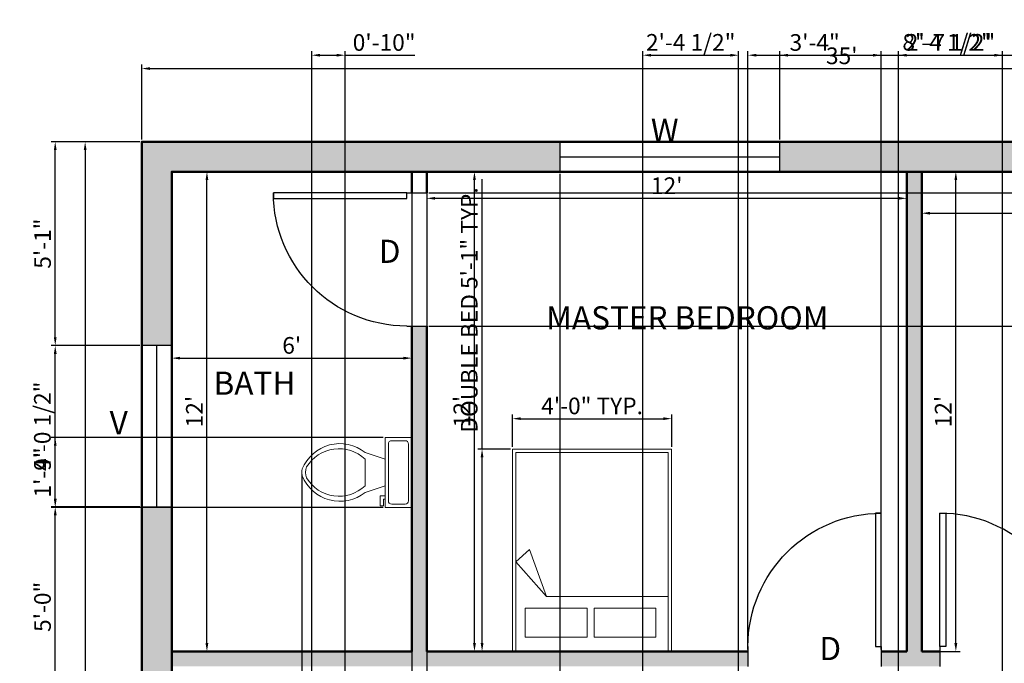
# Model space of a CAD drawing. Units: inches. Extents: x 2168 to 2706, y 2255 to 2760.
# Tile 3 of 4: x 2168 to 2463, y 2567 to 2760. Entities that reach past the tile are written whole.
import ezdxf

# ---------------------------------------------------------------- set-up
doc = ezdxf.new("R2010")
doc.units = ezdxf.units.IN
for name, color, linetype, lineweight in [('A-ANNO-DIMS', 220, 'Continuous', 18), ('A-ANNO-TEXT', 220, 'Continuous', 25), ('A-AREA-IDEN', 220, 'Continuous', 25), ('A-FLOR-FIXT', 9, 'Continuous', 18), ('A-WALL-PATT', 140, 'Continuous', 13), ('DOOR', 30, 'Continuous', 25), ('FUR', 112, 'Continuous', 18), ('WALL', 140, 'Continuous', 50), ('WINDOW', 200, 'Continuous', 25)]:
    doc.layers.add(name, color=color, linetype=linetype, lineweight=lineweight)
doc.styles.get("Standard").update_dxf_attribs({"font": 'arial.ttf'})
doc.dimstyles.new('ISO-25', dxfattribs={"dimtxt": 5, "dimasz": 2.5, "dimexe": 1.25, "dimexo": 0.625, "dimtad": 1, "dimlunit": 4, "dimtxsty": 'Standard', "dimcen": 2.5, "dimadec": 0, "dimazin": 0, "dimtfac": 1, "dimtmove": 0, "dimatfit": 3, "dimfxl": 1, "dimarcsym": 0})

# ---------------------------------------------------------------- blocks, each defined once
blk = doc.blocks.new('*U2')
for p, q in [((0, 0), (0, -6)), ((40, 0), (40, -6))]:
    blk.add_line(p, q)
blk.add_lwpolyline([(0, 0), (0, 40), (1.75, 40), (1.75, 0)], close=True)
blk.add_arc((0, 0), 40, 0, 90)
blk = doc.blocks.new('*U4')
for p, q in [((9.5, -6), (9.5, -2)), ((-10, -8.5), (-8, -8.5)), ((-10, -9.5), (-10, -8.5)), ((-8, -8.5), (-8, -8)), ((-7, -8), (-7, -9.5)), ((-4, -8), (-6, -14)), ((4, -8), (6, -14)), ((-7, -9.5), (-10, -9.5)), ((4, -14), (-4, -14))]:
    blk.add_line(p, q)
blk.add_lwpolyline([(10.5, -8), (10.5, 0), (-10.5, 0), (-10.5, -8)], close=True)
for points in [[(-9.5, -2), (-9.5, -6)], [(8.5, -1), (-8.5, -1)], [(-8.5, -7), (8.5, -7)]]:
    blk.add_lwpolyline(points)
for centre, radius, start, end in [((-8.62, -1.88), 0.884, 81.8699, 188.1301), ((8.62, -1.88), 0.884, 351.8699, 98.1301), ((-8.62, -6.12), 0.884, 171.8699, 278.1301), ((8.62, -6.12), 0.884, 261.8699, 8.1301), ((3.52, -21.58), 12.17, 141.4691, 247.9714), ((4.2, -21.82), 11.33, 136.3677, 238.9468), ((-3.52, -21.58), 12.17, 292.0284, 38.5307), ((-4.2, -21.82), 11.33, 301.053, 43.6321), ((0, -27.88), 4, 245.7318, 294.2682), ((0, -29), 4, 254.8605, 285.1395)]:
    blk.add_arc(centre, radius, start, end)
blk = doc.blocks.new('*D5')
at = {"layer": 'A-ANNO-DIMS', "color": 0, "lineweight": -2, "transparency": 16777216}
for p, q in [((2213.72, 2713.72), (2213.72, 2657.14)), ((2285.72, 2713.72), (2285.72, 2657.14)), ((2216.22, 2658.39), (2283.22, 2658.39))]:
    blk.add_line(p, q, dxfattribs=at)
at = {"layer": 'A-ANNO-DIMS', "color": 0, "transparency": 16777216}
for points in [[(2216.22, 2658.8), (2216.22, 2657.97), (2213.72, 2658.39)], [(2283.22, 2658.8), (2283.22, 2657.97), (2285.72, 2658.39)]]:
    blk.add_solid(points, dxfattribs=at)
at = {"layer": 'Defpoints', "color": 0, "transparency": 16777216}
for p in [(2213.72, 2714.35), (2285.72, 2714.35), (2285.72, 2658.39)]:
    blk.add_point(p, dxfattribs=at)
at = {"layer": 'A-ANNO-DIMS', "color": 0, "transparency": 16777216, "insert": (2249.72, 2661.56), "char_height": 5, "attachment_point": 5}
blk.add_mtext("6'", dxfattribs=at)
blk = doc.blocks.new('*D6')
at = {"layer": 'A-ANNO-DIMS', "color": 0, "lineweight": -2, "transparency": 16777216}
for p, q in [((2214.35, 2714.35), (2225.53, 2714.35)), ((2224.28, 2572.85), (2224.28, 2711.85)), ((2214.35, 2570.35), (2225.53, 2570.35))]:
    blk.add_line(p, q, dxfattribs=at)
at = {"layer": 'A-ANNO-DIMS', "color": 0, "transparency": 16777216}
for points in [[(2223.86, 2711.85), (2224.7, 2711.85), (2224.28, 2714.35)], [(2223.86, 2572.85), (2224.7, 2572.85), (2224.28, 2570.35)]]:
    blk.add_solid(points, dxfattribs=at)
at = {"layer": 'Defpoints', "color": 0, "transparency": 16777216}
for p in [(2213.72, 2714.35), (2224.28, 2714.35), (2213.72, 2570.35)]:
    blk.add_point(p, dxfattribs=at)
at = {"layer": 'A-ANNO-DIMS', "color": 0, "transparency": 16777216, "insert": (2221.15, 2642.35), "char_height": 5, "attachment_point": 5, "rotation": 90}
blk.add_mtext("12'", dxfattribs=at)
blk = doc.blocks.new('*D7')
at = {"layer": 'A-ANNO-DIMS', "color": 0, "lineweight": -2, "transparency": 16777216}
for p, q in [((2290.22, 2713.72), (2290.22, 2705.1)), ((2434.22, 2713.72), (2434.22, 2705.1)), ((2292.72, 2706.35), (2431.72, 2706.35))]:
    blk.add_line(p, q, dxfattribs=at)
at = {"layer": 'A-ANNO-DIMS', "color": 0, "transparency": 16777216}
for points in [[(2292.72, 2706.77), (2292.72, 2705.93), (2290.22, 2706.35)], [(2431.72, 2706.77), (2431.72, 2705.93), (2434.22, 2706.35)]]:
    blk.add_solid(points, dxfattribs=at)
at = {"layer": 'Defpoints', "color": 0, "transparency": 16777216}
for p in [(2290.22, 2714.35), (2434.22, 2714.35), (2434.22, 2706.35)]:
    blk.add_point(p, dxfattribs=at)
at = {"layer": 'A-ANNO-DIMS', "color": 0, "transparency": 16777216, "insert": (2362.22, 2709.49), "char_height": 5, "attachment_point": 5}
blk.add_mtext("12'", dxfattribs=at)
blk = doc.blocks.new('*D8')
at = {"layer": 'A-ANNO-DIMS', "color": 0, "lineweight": -2, "transparency": 16777216}
for p, q in [((2290.85, 2714.35), (2305.79, 2714.35)), ((2304.54, 2572.85), (2304.54, 2711.85)), ((2290.85, 2570.35), (2305.79, 2570.35))]:
    blk.add_line(p, q, dxfattribs=at)
at = {"layer": 'A-ANNO-DIMS', "color": 0, "transparency": 16777216}
for points in [[(2304.12, 2711.85), (2304.95, 2711.85), (2304.54, 2714.35)], [(2304.12, 2572.85), (2304.95, 2572.85), (2304.54, 2570.35)]]:
    blk.add_solid(points, dxfattribs=at)
at = {"layer": 'Defpoints', "color": 0, "transparency": 16777216}
for p in [(2290.22, 2714.35), (2304.54, 2714.35), (2290.22, 2570.35)]:
    blk.add_point(p, dxfattribs=at)
at = {"layer": 'A-ANNO-DIMS', "color": 0, "transparency": 16777216, "insert": (2301.4, 2642.35), "char_height": 5, "attachment_point": 5, "rotation": 90}
blk.add_mtext("12'", dxfattribs=at)
blk = doc.blocks.new('*D9')
at = {"layer": 'A-ANNO-DIMS', "color": 0, "lineweight": -2, "transparency": 16777216}
for p, q in [((2438.72, 2713.72), (2438.72, 2700.63)), ((2615.72, 2713.72), (2615.72, 2700.63)), ((2441.22, 2701.88), (2613.22, 2701.88))]:
    blk.add_line(p, q, dxfattribs=at)
at = {"layer": 'A-ANNO-DIMS', "color": 0, "transparency": 16777216}
for points in [[(2441.22, 2702.3), (2441.22, 2701.46), (2438.72, 2701.88)], [(2613.22, 2702.3), (2613.22, 2701.46), (2615.72, 2701.88)]]:
    blk.add_solid(points, dxfattribs=at)
at = {"layer": 'Defpoints', "color": 0, "transparency": 16777216}
for p in [(2438.72, 2714.35), (2615.72, 2714.35), (2615.72, 2701.88)]:
    blk.add_point(p, dxfattribs=at)
at = {"layer": 'A-ANNO-DIMS', "color": 0, "transparency": 16777216, "insert": (2527.22, 2705.06), "char_height": 5, "attachment_point": 5}
blk.add_mtext('14\'-9"', dxfattribs=at)
blk = doc.blocks.new('*D10')
at = {"layer": 'A-ANNO-DIMS', "color": 0, "lineweight": -2, "transparency": 16777216}
for p, q in [((2439.35, 2714.35), (2450.2, 2714.35)), ((2448.95, 2572.85), (2448.95, 2711.85)), ((2439.35, 2570.35), (2450.2, 2570.35))]:
    blk.add_line(p, q, dxfattribs=at)
at = {"layer": 'A-ANNO-DIMS', "color": 0, "transparency": 16777216}
for points in [[(2448.53, 2711.85), (2449.37, 2711.85), (2448.95, 2714.35)], [(2448.53, 2572.85), (2449.37, 2572.85), (2448.95, 2570.35)]]:
    blk.add_solid(points, dxfattribs=at)
at = {"layer": 'Defpoints', "color": 0, "transparency": 16777216}
for p in [(2438.72, 2714.35), (2448.95, 2714.35), (2438.72, 2570.35)]:
    blk.add_point(p, dxfattribs=at)
at = {"layer": 'A-ANNO-DIMS', "color": 0, "transparency": 16777216, "insert": (2445.81, 2642.35), "char_height": 5, "attachment_point": 5, "rotation": 90}
blk.add_mtext("12'", dxfattribs=at)
blk = doc.blocks.new('*D29')
at = {"layer": 'A-ANNO-DIMS', "color": 0, "lineweight": -2, "transparency": 16777216}
for p, q in [((2204.72, 2723.97), (2204.72, 2746.55)), ((2207.22, 2745.3), (2622.22, 2745.3)), ((2624.72, 2723.97), (2624.72, 2746.55))]:
    blk.add_line(p, q, dxfattribs=at)
at = {"layer": 'A-ANNO-DIMS', "color": 0, "transparency": 16777216}
for points in [[(2207.22, 2745.71), (2207.22, 2744.88), (2204.72, 2745.3)], [(2622.22, 2745.71), (2622.22, 2744.88), (2624.72, 2745.3)]]:
    blk.add_solid(points, dxfattribs=at)
at = {"layer": 'Defpoints', "color": 0, "transparency": 16777216}
for p in [(2624.72, 2745.3), (2204.72, 2723.35), (2624.72, 2723.35)]:
    blk.add_point(p, dxfattribs=at)
at = {"layer": 'A-ANNO-DIMS', "color": 0, "transparency": 16777216, "insert": (2414.72, 2748.48), "char_height": 5, "attachment_point": 5}
blk.add_mtext("35'", dxfattribs=at)
blk = doc.blocks.new('*D30')
at = {"layer": 'A-ANNO-DIMS', "color": 0, "lineweight": -2, "transparency": 16777216}
for p, q in [((2204.1, 2723.35), (2186.49, 2723.35)), ((2187.74, 2720.85), (2187.74, 2305.85)), ((2204.1, 2303.35), (2186.49, 2303.35))]:
    blk.add_line(p, q, dxfattribs=at)
at = {"layer": 'A-ANNO-DIMS', "color": 0, "transparency": 16777216}
for points in [[(2187.33, 2720.85), (2188.16, 2720.85), (2187.74, 2723.35)], [(2187.33, 2305.85), (2188.16, 2305.85), (2187.74, 2303.35)]]:
    blk.add_solid(points, dxfattribs=at)
at = {"layer": 'Defpoints', "color": 0, "transparency": 16777216}
for p in [(2204.72, 2723.35), (2187.74, 2303.35), (2204.72, 2303.35)]:
    blk.add_point(p, dxfattribs=at)
at = {"layer": 'A-ANNO-DIMS', "color": 0, "transparency": 16777216, "insert": (2184.56, 2513.35), "char_height": 5, "attachment_point": 5, "rotation": 90}
blk.add_mtext("35'", dxfattribs=at)
blk = doc.blocks.new('BED-DOUBLE')
for p, q in [((0, 26.86), (4.14, 30.57)), ((4.14, 30.57), (9.23, 16.54)), ((9.23, 16.54), (0, 26.86)), ((45.76, 16.54), (9.23, 16.54))]:
    blk.add_line(p, q)
blk.add_lwpolyline([(46.76, 0), (46.76, 60.76), (-1, 60.76), (-1, 0)])
for points in [[(0, 0), (45.76, 0), (45.76, 59.76), (0, 59.76)], [(2.85, 4.25), (21.39, 4.25), (21.39, 13.05), (2.85, 13.05)], [(23.51, 4.25), (42.05, 4.25), (42.05, 13.05), (23.51, 13.05)]]:
    blk.add_lwpolyline(points, close=True)
blk = doc.blocks.new('WIN-66IN')
blk.add_line((0, 0), (66.01, 0))
blk.add_lwpolyline([(0, -4.5), (66.01, -4.5), (66.01, 4.5), (0, 4.5)], close=True)
blk = doc.blocks.new('*D36')
at = {"layer": 'A-ANNO-DIMS', "color": 0, "lineweight": -2, "transparency": 16777216}
for p, q in [((2306.82, 2631.11), (2306.82, 2712.06)), ((2315.31, 2631.11), (2305.57, 2631.11)), ((2306.82, 2572.85), (2306.82, 2628.61)), ((2315.31, 2570.35), (2305.57, 2570.35))]:
    blk.add_line(p, q, dxfattribs=at)
at = {"layer": 'A-ANNO-DIMS', "color": 0, "transparency": 16777216}
for points in [[(2306.4, 2628.61), (2307.24, 2628.61), (2306.82, 2631.11)], [(2306.4, 2572.85), (2307.24, 2572.85), (2306.82, 2570.35)]]:
    blk.add_solid(points, dxfattribs=at)
at = {"layer": 'Defpoints', "color": 0, "transparency": 16777216}
for p in [(2306.82, 2631.11), (2315.94, 2631.11), (2315.94, 2570.35)]:
    blk.add_point(p, dxfattribs=at)
at = {"layer": 'A-ANNO-DIMS', "color": 0, "transparency": 16777216, "insert": (2303.61, 2672.83), "char_height": 5, "attachment_point": 5, "rotation": 90}
blk.add_mtext('DOUBLE BED 5\'-1" TYP.', dxfattribs=at)
blk = doc.blocks.new('*D37')
at = {"layer": 'A-ANNO-DIMS', "color": 0, "lineweight": -2, "transparency": 16777216}
for p, q in [((2315.94, 2631.74), (2315.94, 2641.47)), ((2363.7, 2631.74), (2363.7, 2641.47)), ((2318.44, 2640.22), (2361.2, 2640.22))]:
    blk.add_line(p, q, dxfattribs=at)
at = {"layer": 'A-ANNO-DIMS', "color": 0, "transparency": 16777216}
for points in [[(2318.44, 2640.64), (2318.44, 2639.81), (2315.94, 2640.22)], [(2361.2, 2640.64), (2361.2, 2639.81), (2363.7, 2640.22)]]:
    blk.add_solid(points, dxfattribs=at)
at = {"layer": 'Defpoints', "color": 0, "transparency": 16777216}
for p in [(2363.7, 2640.22), (2315.94, 2631.11), (2363.7, 2631.11)]:
    blk.add_point(p, dxfattribs=at)
at = {"layer": 'A-ANNO-DIMS', "color": 0, "transparency": 16777216, "insert": (2339.82, 2643.4), "char_height": 5, "attachment_point": 5}
blk.add_mtext('4\'-0" TYP.', dxfattribs=at)
blk = doc.blocks.new('*D47')
at = {"layer": 'A-ANNO-DIMS', "color": 0, "lineweight": -2, "transparency": 16777216}
for p, q in [((2386.59, 2570.97), (2386.59, 2750.55)), ((2426.59, 2570.97), (2426.59, 2750.55)), ((2389.09, 2749.3), (2424.09, 2749.3))]:
    blk.add_line(p, q, dxfattribs=at)
at = {"layer": 'A-ANNO-DIMS', "color": 0, "transparency": 16777216}
for points in [[(2389.09, 2749.71), (2389.09, 2748.88), (2386.59, 2749.3)], [(2424.09, 2749.71), (2424.09, 2748.88), (2426.59, 2749.3)]]:
    blk.add_solid(points, dxfattribs=at)
at = {"layer": 'Defpoints', "color": 0, "transparency": 16777216}
for p in [(2426.59, 2749.3), (2386.59, 2570.35), (2426.59, 2570.35)]:
    blk.add_point(p, dxfattribs=at)
at = {"layer": 'A-ANNO-DIMS', "color": 0, "transparency": 16777216, "insert": (2406.59, 2752.48), "char_height": 5, "attachment_point": 5}
blk.add_mtext('3\'-4"', dxfattribs=at)
blk = doc.blocks.new('*D49')
at = {"layer": 'A-ANNO-DIMS', "color": 0, "lineweight": -2, "transparency": 16777216}
for p, q in [((2355.04, 2389.47), (2355.04, 2750.55)), ((2383.78, 2389.47), (2383.78, 2750.55)), ((2357.54, 2749.3), (2381.28, 2749.3))]:
    blk.add_line(p, q, dxfattribs=at)
at = {"layer": 'A-ANNO-DIMS', "color": 0, "transparency": 16777216}
for points in [[(2357.54, 2749.71), (2357.54, 2748.88), (2355.04, 2749.3)], [(2381.28, 2749.71), (2381.28, 2748.88), (2383.78, 2749.3)]]:
    blk.add_solid(points, dxfattribs=at)
at = {"layer": 'Defpoints', "color": 0, "transparency": 16777216}
for p in [(2383.78, 2749.3), (2355.04, 2388.85), (2383.78, 2388.85)]:
    blk.add_point(p, dxfattribs=at)
at = {"layer": 'A-ANNO-DIMS', "color": 0, "transparency": 16777216, "insert": (2369.41, 2752.51), "char_height": 5, "attachment_point": 5}
blk.add_mtext('2\'-4 1/2"', dxfattribs=at)
blk = doc.blocks.new('*D53')
at = {"layer": 'A-ANNO-DIMS', "color": 0, "lineweight": -2, "transparency": 16777216}
for p, q in [((2431.71, 2524.6), (2431.71, 2750.55)), ((2462.98, 2524.6), (2462.98, 2750.55)), ((2434.21, 2749.3), (2460.48, 2749.3))]:
    blk.add_line(p, q, dxfattribs=at)
at = {"layer": 'A-ANNO-DIMS', "color": 0, "transparency": 16777216}
for points in [[(2434.21, 2749.71), (2434.21, 2748.88), (2431.71, 2749.3)], [(2460.48, 2749.71), (2460.48, 2748.88), (2462.98, 2749.3)]]:
    blk.add_solid(points, dxfattribs=at)
at = {"layer": 'Defpoints', "color": 0, "transparency": 16777216}
for p in [(2462.98, 2749.3), (2431.71, 2523.98), (2462.98, 2523.98)]:
    blk.add_point(p, dxfattribs=at)
at = {"layer": 'A-ANNO-DIMS', "color": 0, "transparency": 16777216, "insert": (2447.34, 2752.51), "char_height": 5, "attachment_point": 5}
blk.add_mtext('2\'-7 1/2"', dxfattribs=at)
blk = doc.blocks.new('*D64')
at = {"layer": 'A-ANNO-DIMS', "color": 0, "lineweight": -2, "transparency": 16777216}
for p, q in [((2290.22, 2713.72), (2290.22, 2276.15)), ((2330.12, 2713.72), (2330.12, 2276.15)), ((2292.72, 2277.4), (2327.62, 2277.4))]:
    blk.add_line(p, q, dxfattribs=at)
at = {"layer": 'A-ANNO-DIMS', "color": 0, "transparency": 16777216}
for points in [[(2292.72, 2277.81), (2292.72, 2276.98), (2290.22, 2277.4)], [(2327.62, 2277.81), (2327.62, 2276.98), (2330.12, 2277.4)]]:
    blk.add_solid(points, dxfattribs=at)
at = {"layer": 'Defpoints', "color": 0, "transparency": 16777216}
for p in [(2290.22, 2714.35), (2330.12, 2714.35), (2330.12, 2277.4)]:
    blk.add_point(p, dxfattribs=at)
at = {"layer": 'A-ANNO-DIMS', "color": 0, "transparency": 16777216, "insert": (2310.17, 2280.58), "char_height": 5, "attachment_point": 5}
blk.add_mtext('3\'-4"', dxfattribs=at)
blk = doc.blocks.new('*D65')
at = {"layer": 'A-ANNO-DIMS', "color": 0, "lineweight": -2, "transparency": 16777216}
for p, q in [((2396.13, 2723.97), (2396.13, 2750.55)), ((2496.54, 2723.97), (2496.54, 2750.55)), ((2398.63, 2749.3), (2494.04, 2749.3))]:
    blk.add_line(p, q, dxfattribs=at)
at = {"layer": 'A-ANNO-DIMS', "color": 0, "transparency": 16777216}
for points in [[(2398.63, 2749.71), (2398.63, 2748.88), (2396.13, 2749.3)], [(2494.04, 2749.71), (2494.04, 2748.88), (2496.54, 2749.3)]]:
    blk.add_solid(points, dxfattribs=at)
at = {"layer": 'Defpoints', "color": 0, "transparency": 16777216}
for p in [(2496.54, 2749.3), (2396.13, 2723.35), (2496.54, 2723.35)]:
    blk.add_point(p, dxfattribs=at)
at = {"layer": 'A-ANNO-DIMS', "color": 0, "transparency": 16777216, "insert": (2446.33, 2752.51), "char_height": 5, "attachment_point": 5}
blk.add_mtext('8\'-4 1/2"', dxfattribs=at)
blk = doc.blocks.new('*D68')
at = {"layer": 'A-ANNO-DIMS', "color": 0, "lineweight": -2, "transparency": 16777216}
for p, q in [((2204.1, 2662.15), (2177.52, 2662.15)), ((2178.77, 2616.23), (2178.77, 2659.65)), ((2204.1, 2613.73), (2177.52, 2613.73))]:
    blk.add_line(p, q, dxfattribs=at)
at = {"layer": 'A-ANNO-DIMS', "color": 0, "transparency": 16777216}
for points in [[(2178.36, 2659.65), (2179.19, 2659.65), (2178.77, 2662.15)], [(2178.36, 2616.23), (2179.19, 2616.23), (2178.77, 2613.73)]]:
    blk.add_solid(points, dxfattribs=at)
at = {"layer": 'Defpoints', "color": 0, "transparency": 16777216}
for p in [(2178.77, 2662.15), (2204.72, 2662.15), (2204.72, 2613.73)]:
    blk.add_point(p, dxfattribs=at)
at = {"layer": 'A-ANNO-DIMS', "color": 0, "transparency": 16777216, "insert": (2175.56, 2637.94), "char_height": 5, "attachment_point": 5, "rotation": 90}
blk.add_mtext('4\'-0 1/2"', dxfattribs=at)
blk = doc.blocks.new('*D69')
at = {"layer": 'A-ANNO-DIMS', "color": 0, "lineweight": -2, "transparency": 16777216}
for p, q in [((2204.1, 2723.35), (2177.52, 2723.35)), ((2178.77, 2664.65), (2178.77, 2720.85)), ((2204.1, 2662.15), (2177.52, 2662.15))]:
    blk.add_line(p, q, dxfattribs=at)
at = {"layer": 'A-ANNO-DIMS', "color": 0, "transparency": 16777216}
for points in [[(2178.36, 2720.85), (2179.19, 2720.85), (2178.77, 2723.35)], [(2178.36, 2664.65), (2179.19, 2664.65), (2178.77, 2662.15)]]:
    blk.add_solid(points, dxfattribs=at)
at = {"layer": 'Defpoints', "color": 0, "transparency": 16777216}
for p in [(2178.77, 2723.35), (2204.72, 2723.35), (2204.72, 2662.15)]:
    blk.add_point(p, dxfattribs=at)
at = {"layer": 'A-ANNO-DIMS', "color": 0, "transparency": 16777216, "insert": (2175.6, 2692.75), "char_height": 5, "attachment_point": 5, "rotation": 90}
blk.add_mtext('5\'-1"', dxfattribs=at)
blk = doc.blocks.new('*D71')
at = {"layer": 'A-ANNO-DIMS', "color": 0, "lineweight": -2, "transparency": 16777216}
for p, q in [((2204.1, 2613.73), (2177.52, 2613.73)), ((2178.77, 2556.26), (2178.77, 2611.23)), ((2204.1, 2553.76), (2177.52, 2553.76))]:
    blk.add_line(p, q, dxfattribs=at)
at = {"layer": 'A-ANNO-DIMS', "color": 0, "transparency": 16777216}
for points in [[(2178.36, 2611.23), (2179.19, 2611.23), (2178.77, 2613.73)], [(2178.36, 2556.26), (2179.19, 2556.26), (2178.77, 2553.76)]]:
    blk.add_solid(points, dxfattribs=at)
at = {"layer": 'Defpoints', "color": 0, "transparency": 16777216}
for p in [(2178.77, 2613.73), (2204.72, 2613.73), (2204.72, 2553.76)]:
    blk.add_point(p, dxfattribs=at)
at = {"layer": 'A-ANNO-DIMS', "color": 0, "transparency": 16777216, "insert": (2175.6, 2583.75), "char_height": 5, "attachment_point": 5, "rotation": 90}
blk.add_mtext('5\'-0"', dxfattribs=at)
blk = doc.blocks.new('*D74')
at = {"layer": 'A-ANNO-DIMS', "color": 0, "lineweight": -2, "transparency": 16777216}
for p, q in [((2255.72, 2525.22), (2255.72, 2750.55)), ((2265.72, 2525.22), (2265.72, 2750.55)), ((2258.22, 2749.3), (2263.22, 2749.3)), ((2265.72, 2749.3), (2286.65, 2749.3))]:
    blk.add_line(p, q, dxfattribs=at)
at = {"layer": 'A-ANNO-DIMS', "color": 0, "transparency": 16777216}
for points in [[(2258.22, 2749.71), (2258.22, 2748.88), (2255.72, 2749.3)], [(2263.22, 2749.71), (2263.22, 2748.88), (2265.72, 2749.3)]]:
    blk.add_solid(points, dxfattribs=at)
at = {"layer": 'Defpoints', "color": 0, "transparency": 16777216}
for p in [(2265.72, 2749.3), (2255.72, 2524.6), (2265.72, 2524.6)]:
    blk.add_point(p, dxfattribs=at)
at = {"layer": 'A-ANNO-DIMS', "color": 0, "transparency": 16777216, "insert": (2277.44, 2752.47), "char_height": 5, "attachment_point": 5}
blk.add_mtext('0\'-10"', dxfattribs=at)
blk = doc.blocks.new('*D75')
at = {"layer": 'A-ANNO-DIMS', "color": 0, "lineweight": -2, "transparency": 16777216}
for p, q in [((2277.1, 2634.58), (2177.52, 2634.58)), ((2178.77, 2616.08), (2178.77, 2632.08)), ((2277.1, 2613.58), (2177.52, 2613.58))]:
    blk.add_line(p, q, dxfattribs=at)
at = {"layer": 'A-ANNO-DIMS', "color": 0, "transparency": 16777216}
for points in [[(2178.36, 2632.08), (2179.19, 2632.08), (2178.77, 2634.58)], [(2178.36, 2616.08), (2179.19, 2616.08), (2178.77, 2613.58)]]:
    blk.add_solid(points, dxfattribs=at)
at = {"layer": 'Defpoints', "color": 0, "transparency": 16777216}
for p in [(2178.77, 2634.58), (2277.72, 2634.58), (2277.72, 2613.58)]:
    blk.add_point(p, dxfattribs=at)
at = {"layer": 'A-ANNO-DIMS', "color": 0, "transparency": 16777216, "insert": (2175.6, 2624.08), "char_height": 5, "attachment_point": 5, "rotation": 90}
blk.add_mtext('1\'-9"', dxfattribs=at)
blk = doc.blocks.new('*D76')
at = {"layer": 'A-ANNO-DIMS', "color": 0, "lineweight": -2, "transparency": 16777216}
for p, q in [((2252.72, 2623.46), (2252.72, 2276.15)), ((2285.72, 2612.95), (2285.72, 2276.15)), ((2255.22, 2277.4), (2283.22, 2277.4))]:
    blk.add_line(p, q, dxfattribs=at)
at = {"layer": 'A-ANNO-DIMS', "color": 0, "transparency": 16777216}
for points in [[(2255.22, 2277.81), (2255.22, 2276.98), (2252.72, 2277.4)], [(2283.22, 2277.81), (2283.22, 2276.98), (2285.72, 2277.4)]]:
    blk.add_solid(points, dxfattribs=at)
at = {"layer": 'Defpoints', "color": 0, "transparency": 16777216}
for p in [(2252.72, 2624.08), (2285.72, 2613.58), (2285.72, 2277.4)]:
    blk.add_point(p, dxfattribs=at)
at = {"layer": 'A-ANNO-DIMS', "color": 0, "transparency": 16777216, "insert": (2269.22, 2280.57), "char_height": 5, "attachment_point": 5}
blk.add_mtext('2\'-9"', dxfattribs=at)
blk = doc.blocks.new('*D77')
at = {"layer": 'A-ANNO-DIMS', "color": 0, "lineweight": -2, "transparency": 16777216}
for p, q in [((2290.85, 2708.02), (2702.92, 2708.02)), ((2701.67, 2670.52), (2701.67, 2705.52)), ((2290.85, 2668.02), (2702.92, 2668.02))]:
    blk.add_line(p, q, dxfattribs=at)
at = {"layer": 'A-ANNO-DIMS', "color": 0, "transparency": 16777216}
for points in [[(2701.26, 2705.52), (2702.09, 2705.52), (2701.67, 2708.02)], [(2701.26, 2670.52), (2702.09, 2670.52), (2701.67, 2668.02)]]:
    blk.add_solid(points, dxfattribs=at)
at = {"layer": 'Defpoints', "color": 0, "transparency": 16777216}
for p in [(2290.22, 2708.02), (2701.67, 2708.02), (2290.22, 2668.02)]:
    blk.add_point(p, dxfattribs=at)
at = {"layer": 'A-ANNO-DIMS', "color": 0, "transparency": 16777216, "insert": (2698.49, 2688.02), "char_height": 5, "attachment_point": 5, "rotation": 90}
blk.add_mtext('3\'-4"', dxfattribs=at)

msp = doc.modelspace()

# ---------------------------------------------------------------- hatches: boundary and pattern name
at = {"layer": 'A-WALL-PATT'}
h = msp.add_hatch(color=256, dxfattribs=at)
h.dxf.hatch_style = 1
h.paths.add_polyline_path([(2330.12, 2723.347), (2204.724, 2723.347), (2204.724, 2662.147), (2213.724, 2662.147), (2213.724, 2714.347), (2285.724, 2714.347), (2330.12, 2714.347)])
h.paths.add_polyline_path([(2496.542, 2723.347), (2396.128, 2723.347), (2396.128, 2714.347), (2434.224, 2714.347), (2496.542, 2714.347)])
h.paths.add_polyline_path([(2624.724, 2723.347), (2562.55, 2723.347), (2562.55, 2714.347), (2615.724, 2714.347), (2615.724, 2545.448), (2624.724, 2545.448)])
h.paths.add_polyline_path([(2438.724, 2714.347), (2434.224, 2714.347), (2434.224, 2570.347), (2426.591, 2570.347), (2426.591, 2565.847), (2438.724, 2565.847), (2444.149, 2565.847), (2444.149, 2570.347), (2438.724, 2570.347)])
h.paths.add_polyline_path([(2290.224, 2668.023), (2285.724, 2668.023), (2285.724, 2570.347), (2213.724, 2570.347), (2213.724, 2565.847), (2290.224, 2565.847), (2386.591, 2565.847), (2386.591, 2570.347), (2290.224, 2570.347)])
h.paths.add_polyline_path([(2514.678, 2570.347), (2514.678, 2630.11), (2560.439, 2630.11), (2560.439, 2570.347)], flags=16)
h.paths.add_polyline_path([(2517.528, 2574.595), (2517.528, 2583.399), (2536.063, 2583.399), (2536.063, 2574.595)], flags=0)
h.paths.add_polyline_path([(2523.909, 2586.89), (2514.678, 2597.212), (2518.822, 2600.918)], flags=0)
h.paths.add_polyline_path([(2538.189, 2574.595), (2538.189, 2583.399), (2556.724, 2583.399), (2556.724, 2574.595)], flags=0)
h.paths.add_polyline_path([(2560.439, 2630.11), (2560.439, 2570.347), (2514.678, 2570.347), (2514.678, 2630.11)])
h.paths.add_polyline_path([(2213.724, 2389.588), (2204.724, 2389.588), (2204.724, 2303.347), (2229.06, 2303.347), (2229.06, 2312.347), (2213.724, 2312.347)])
h.paths.add_polyline_path([(2213.724, 2507.677), (2204.724, 2507.677), (2204.724, 2462.696), (2213.724, 2462.696)])
h.paths.add_polyline_path([(2204.724, 2553.759), (2213.724, 2553.759), (2213.724, 2613.731), (2204.724, 2613.731)])

# ---------------------------------------------------------------- linework, layer by layer
at = {"layer": 'WALL'}
for p, q in [((2204.724, 2723.347), (2624.724, 2723.347)), ((2204.724, 2303.347), (2204.724, 2723.347)), ((2213.724, 2714.347), (2285.724, 2714.347)), ((2285.724, 2714.347), (2285.724, 2708.023)), ((2290.224, 2714.347), (2290.224, 2708.023)), ((2290.224, 2714.347), (2434.224, 2714.347)), ((2434.224, 2714.347), (2434.224, 2570.347)), ((2438.724, 2714.347), (2438.724, 2570.347)), ((2285.724, 2668.023), (2285.724, 2570.347)), ((2290.224, 2668.023), (2290.224, 2570.347)), ((2285.724, 2570.347), (2213.724, 2570.347)), ((2386.591, 2570.347), (2290.224, 2570.347)), ((2434.224, 2570.347), (2426.591, 2570.347)), ((2438.724, 2570.347), (2444.149, 2570.347))]:
    msp.add_line(p, q, dxfattribs=at)
for points in [[(2572.054, 2303.347), (2204.724, 2303.347), (2204.724, 2723.347), (2624.724, 2723.347), (2624.724, 2303.347), (2612.054, 2303.347)], [(2572.166, 2312.347), (2213.724, 2312.347), (2213.724, 2714.347), (2615.724, 2714.347), (2615.724, 2312.347), (2610.304, 2312.347)]]:
    msp.add_lwpolyline(points, dxfattribs=at)
at = {"layer": 'WINDOW'}
msp.add_line((2209.224, 2613.731), (2209.224, 2662.147), dxfattribs=at)
msp.add_lwpolyline([(2213.724, 2662.147), (2204.724, 2662.147), (2204.724, 2613.731), (2213.724, 2613.731)], close=True, dxfattribs=at)

# ---------------------------------------------------------------- block references
at = {"layer": 'A-FLOR-FIXT', "xscale": -1, "rotation": 270}
msp.add_blockref('*U4', (2285.724, 2624.08), dxfattribs=at)
at = {"layer": 'DOOR', "xscale": -1, "rotation": 90}
msp.add_blockref('*U2', (2284.224, 2708.023), dxfattribs=at)
at = {"layer": 'DOOR', "xscale": -1}
msp.add_blockref('*U2', (2426.591, 2571.847), dxfattribs=at)
at = {"layer": 'DOOR'}
msp.add_blockref('*U2', (2444.149, 2571.847), dxfattribs=at)
at = {"layer": 'FUR'}
msp.add_blockref('BED-DOUBLE', (2316.936, 2570.347), dxfattribs=at)
at = {"layer": 'WINDOW'}
msp.add_blockref('WIN-66IN', (2330.12, 2718.847), dxfattribs=at)

# ---------------------------------------------------------------- texts
at = {"layer": 'A-ANNO-TEXT', "char_height": 6.951, "attachment_point": 1}
for s, insert in [('W', (2357.454, 2730.298)), ('D', (2275.821, 2693.919)), ('V', (2195.081, 2642.506)), ('D', (2408.003, 2574.701))]:
    msp.add_mtext_dynamic_manual_height_columns(s, width=121.01281, gutter_width=34.753, heights=[0], dxfattribs=dict(at, insert=insert))
at = {"layer": 'A-AREA-IDEN', "attachment_point": 1}
for s, insert, char_height in [('MASTER BEDROOM', (2326.062, 2673.966), 6.95057), ('BATH', (2226.255, 2654.347), 6.9506)]:
    msp.add_mtext_dynamic_manual_height_columns(s, width=121.01281, gutter_width=34.753, heights=[0], dxfattribs=dict(at, insert=insert, char_height=char_height))

# ---------------------------------------------------------------- dimensions: what is measured, and where the dimension line sits
at = {"layer": 'A-ANNO-DIMS'}
for base, p1, p2, override, picture, middle in [((2383.783, 2749.297), (2355.045, 2388.847), (2383.783, 2388.847), {"dimdec": 1, "dimlfac": 1, "dimrnd": 0, "dimzin": 1, "dimdsep": 46, "dimlunit": 4, "dimfrac": 2}, '*D49', (2369.414, 2752.507)), ((2496.542, 2749.297), (2396.128, 2723.347), (2496.542, 2723.347), {"dimdec": 1, "dimlfac": 1, "dimrnd": 0, "dimzin": 1, "dimdsep": 46, "dimlunit": 4, "dimfrac": 2}, '*D65', (2446.335, 2752.507)), ((2462.979, 2749.297), (2431.708, 2523.979), (2462.979, 2523.979), {"dimdec": 1, "dimlfac": 1, "dimrnd": 0, "dimzin": 1, "dimdsep": 46, "dimlunit": 4, "dimfrac": 2}, '*D53', (2447.344, 2752.507)), ((2265.724, 2749.297), (2255.724, 2524.597), (2265.724, 2524.597), {"dimdec": 1, "dimlfac": 1, "dimrnd": 0, "dimzin": 1, "dimdsep": 46, "dimlunit": 4, "dimfrac": 2}, '*D74', (2277.437, 2752.475)), ((2426.591, 2749.297), (2386.591, 2570.347), (2426.591, 2570.347), {"dimdec": 1, "dimlfac": 1, "dimrnd": 0, "dimzin": 1, "dimdsep": 46, "dimlunit": 4, "dimfrac": 2}, '*D47', (2406.591, 2752.477)), ((2624.724, 2745.296), (2204.724, 2723.347), (2624.724, 2723.347), {"dimclrd": 0, "dimclre": 0, "dimclrt": 0}, '*D29', (2414.724, 2748.475)), ((2285.724, 2658.385), (2213.724, 2714.347), (2285.724, 2714.347), {"dimclrd": 0, "dimclre": 0, "dimclrt": 0}, '*D5', (2249.724, 2661.563)), ((2434.224, 2706.35), (2290.224, 2714.347), (2434.224, 2714.347), {"dimclrd": 0, "dimclre": 0, "dimclrt": 0}, '*D7', (2362.224, 2709.485)), ((2330.12, 2277.397), (2290.224, 2714.347), (2330.12, 2714.347), {"dimdec": 1, "dimlfac": 1, "dimrnd": 0, "dimzin": 1, "dimdsep": 46, "dimlunit": 4, "dimfrac": 2}, '*D64', (2310.172, 2280.577)), ((2615.724, 2701.881), (2438.724, 2714.347), (2615.724, 2714.347), {"dimclrd": 0, "dimclre": 0, "dimclrt": 0}, '*D9', (2527.224, 2705.059)), ((2285.724, 2277.397), (2252.724, 2624.08), (2285.724, 2613.58), {"dimdec": 1, "dimlfac": 1, "dimrnd": 0, "dimzin": 1, "dimdsep": 46, "dimlunit": 4, "dimfrac": 2}, '*D76', (2269.224, 2280.575))]:
    dim = msp.add_linear_dim(base=base, p1=p1, p2=p2, dimstyle='ISO-25', override=override, dxfattribs=at)
    dim.commit()
    dim.dimension.update_dxf_attribs({"geometry": picture, "text_midpoint": middle})
for base, p1, p2, override, picture, middle in [((2178.774, 2723.347), (2204.724, 2662.147), (2204.724, 2723.347), {"dimdec": 1, "dimlfac": 1, "dimrnd": 0, "dimzin": 1, "dimdsep": 46, "dimlunit": 4, "dimfrac": 2}, '*D69', (2175.596, 2692.747)), ((2187.744, 2303.347), (2204.724, 2723.347), (2204.724, 2303.347), {"dimclrd": 0, "dimclre": 0, "dimclrt": 0}, '*D30', (2184.565, 2513.347)), ((2224.28, 2714.347), (2213.724, 2570.347), (2213.724, 2714.347), {"dimclrd": 0, "dimclre": 0, "dimclrt": 0}, '*D6', (2221.145, 2642.347)), ((2304.537, 2714.347), (2290.224, 2570.347), (2290.224, 2714.347), {"dimclrd": 0, "dimclre": 0, "dimclrt": 0}, '*D8', (2301.402, 2642.347)), ((2448.949, 2714.347), (2438.724, 2570.347), (2438.724, 2714.347), {"dimclrd": 0, "dimclre": 0, "dimclrt": 0}, '*D10', (2445.813, 2642.347)), ((2701.674, 2708.023), (2290.224, 2668.023), (2290.224, 2708.023), {"dimdec": 1, "dimlfac": 1, "dimrnd": 0, "dimzin": 1, "dimdsep": 46, "dimlunit": 4, "dimfrac": 2}, '*D77', (2698.494, 2688.023)), ((2178.774, 2662.147), (2204.724, 2613.731), (2204.724, 2662.147), {"dimdec": 1, "dimlfac": 1, "dimrnd": 0, "dimzin": 1, "dimdsep": 46, "dimlunit": 4, "dimfrac": 2}, '*D68', (2175.564, 2637.939)), ((2178.774, 2634.58), (2277.724, 2613.58), (2277.724, 2634.58), {"dimdec": 1, "dimlfac": 1, "dimrnd": 0, "dimzin": 1, "dimdsep": 46, "dimlunit": 4, "dimfrac": 2}, '*D75', (2175.596, 2624.08)), ((2178.774, 2613.731), (2204.724, 2553.759), (2204.724, 2613.731), {"dimdec": 1, "dimlfac": 1, "dimrnd": 0, "dimzin": 1, "dimdsep": 46, "dimlunit": 4, "dimfrac": 2}, '*D71', (2175.596, 2583.745))]:
    dim = msp.add_linear_dim(base=base, p1=p1, p2=p2, angle=90, dimstyle='ISO-25', override=override, dxfattribs=at)
    dim.commit()
    dim.dimension.update_dxf_attribs({"geometry": picture, "text_midpoint": middle})
dim = msp.add_linear_dim(base=(2306.821, 2631.11), p1=(2315.936, 2570.347), p2=(2315.936, 2631.11), angle=90, text='DOUBLE BED <> TYP.', dimstyle='ISO-25', override={"dimdec": 1, "dimlfac": 1, "dimrnd": 0, "dimzin": 1, "dimdsep": 46, "dimlunit": 4, "dimfrac": 2}, dxfattribs=at)
dim.commit()
dim.dimension.update_dxf_attribs({"geometry": '*D36', "text_midpoint": (2303.609, 2672.834)})
dim = msp.add_linear_dim(base=(2363.697, 2640.225), p1=(2315.936, 2631.11), p2=(2363.697, 2631.11), text='<> TYP.', dimstyle='ISO-25', override={"dimdec": 1, "dimlfac": 1, "dimrnd": 0, "dimzin": 1, "dimdsep": 46, "dimlunit": 4, "dimfrac": 2}, dxfattribs=at)
dim.commit()
dim.dimension.update_dxf_attribs({"geometry": '*D37', "text_midpoint": (2339.817, 2643.403)})

doc.saveas('drawing.dxf')
